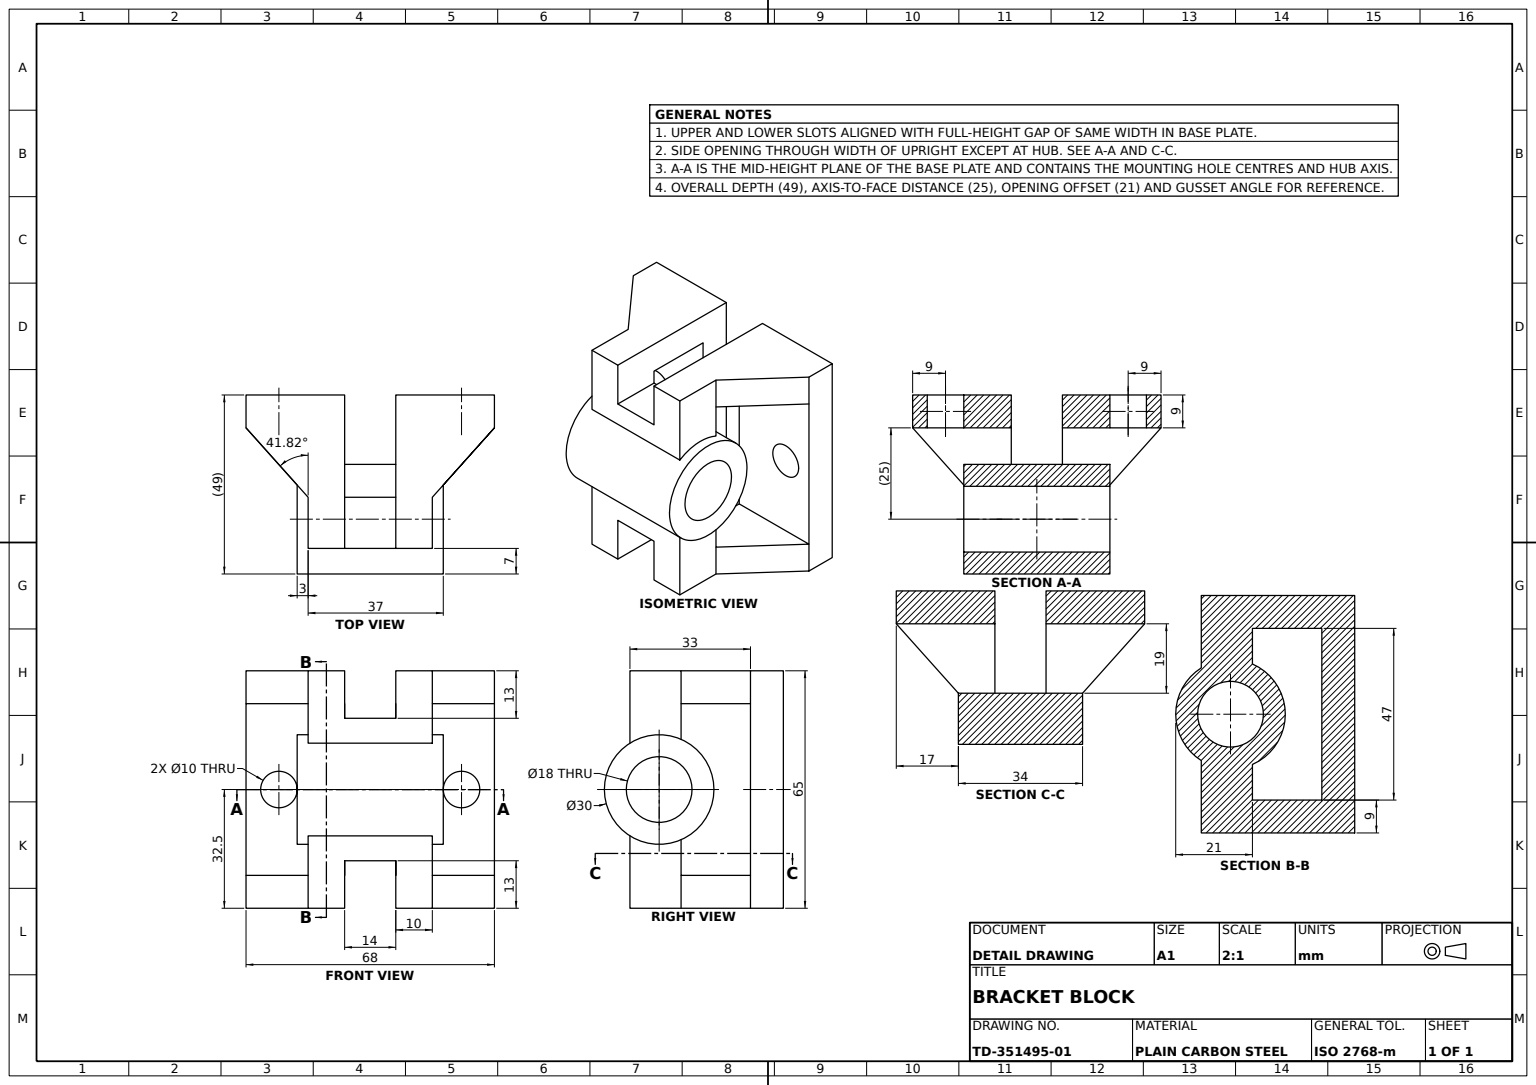
from build123d import *

# Parameters (mm, degrees)
BASE_PLATE_SKETCH_W        = 68
BASE_PLATE_SKETCH_H        = 65
BASE_PLATE_68X65_DEPTH     = 9
UPRIGHT_BLOCK_DEPTH        = 9
SECOND_UPRIGHT_BLOCK_DEPTH = 9
SIDE_WEB_SKETCH_W          = 34
SIDE_WEB_SKETCH_H          = 14
SIDE_WEB_DEPTH             = 65
UPPER_SLOT_7X14_DEPTH      = 13
LOWER_SLOT_7X14_DEPTH      = 13
THROUGH_CHANNEL_SKETCH_W   = 14
THROUGH_CHANNEL_SKETCH_H   = 9
THROUGH_CHANNEL_DEPTH      = 65
BEARING_HUB_SKETCH_R       = 15
BEARING_HUB_DEPTH          = 37
HUB_START                  = 3
HUB_COLLAR_SKETCH_30_R     = 15
HUB_COLLAR_30_DEPTH        = 3
CENTER_BORE_SKETCH_18_R    = 9
CENTER_BORE_18_DEPTH       = 65
SIDE_POCKET_SKETCH_R       = 5
SIDE_POCKET_CUT_DEPTH      = 9


with BuildPart() as part:
    # Base Plate Sketch → Base Plate 68x65 (new body)
    with BuildSketch(Plane.XY):
        with Locations((34, 32.5)):
            Rectangle(BASE_PLATE_SKETCH_W, BASE_PLATE_SKETCH_H)
    extrude(amount=BASE_PLATE_68X65_DEPTH)

    # Upright Block Sketch → Upright Block (add)
    with BuildSketch(Plane.XZ):
        Polygon((0, 9), (68, 9), (51, 28), (51, 42), (34, 42), (17, 42), (17, 28), align=None)
    extrude(amount=-UPRIGHT_BLOCK_DEPTH)

    # Second Upright Sketch → Second Upright Block (add)
    with BuildSketch(Plane(origin=(0, 65, 0), x_dir=(1, 0, 0), z_dir=(0, 1, 0))):
        Polygon((34, -42), (51, -42), (51, -28), (68, -9), (0, -9), (17, -28), (17, -42), align=None)
    extrude(amount=-SECOND_UPRIGHT_BLOCK_DEPTH)

    # Side Web Sketch → Side Web (add)
    with BuildSketch(Plane.XZ):
        with Locations((34, 35)):
            Rectangle(SIDE_WEB_SKETCH_W, SIDE_WEB_SKETCH_H)
    extrude(amount=-SIDE_WEB_DEPTH)

    # Upper Slot Sketch → Upper Slot 7x14 (cut)
    with BuildSketch(Plane.XZ):
        Polygon((34, 42), (41, 42), (41, 0), (27, 0), (27, 42), align=None)
    extrude(amount=-UPPER_SLOT_7X14_DEPTH, mode=Mode.SUBTRACT)

    # Lower Slot Sketch → Lower Slot 7x14 (cut)
    with BuildSketch(Plane(origin=(0, 65, 0), x_dir=(1, 0, 0), z_dir=(0, 1, 0))):
        Polygon((34, -42), (41, -42), (41, 0), (27, 0), (27, -42), align=None)
    extrude(amount=-LOWER_SLOT_7X14_DEPTH, mode=Mode.SUBTRACT)

    # Through Channel Sketch → Through Channel (cut)
    with BuildSketch(Plane.XZ.offset(-13)):
        with Locations((34, 4.5)):
            Rectangle(THROUGH_CHANNEL_SKETCH_W, THROUGH_CHANNEL_SKETCH_H)
    extrude(amount=-THROUGH_CHANNEL_DEPTH, mode=Mode.SUBTRACT)

    # Bearing Hub Sketch → Bearing Hub (add)
    with BuildSketch(Plane.ZY.offset(-17)):
        with Locations((34, 32.5)):
            Circle(BEARING_HUB_SKETCH_R)
    extrude(amount=-BEARING_HUB_DEPTH)

    # Hub Collar Sketch Ø30 → Hub Collar Ø30 (add)
    with BuildSketch(Plane.ZY.offset(-17).offset(HUB_START)):
        with Locations((34, 32.5)):
            Circle(HUB_COLLAR_SKETCH_30_R)
    extrude(amount=-HUB_COLLAR_30_DEPTH)

    # Center Bore Sketch Ø18 → Center Bore Ø18 (cut)
    with BuildSketch(Plane.ZY.offset(-14)):
        with Locations((34, 32.5)):
            Circle(CENTER_BORE_SKETCH_18_R)
    extrude(amount=-CENTER_BORE_18_DEPTH, mode=Mode.SUBTRACT)

    # Side Pocket Sketch → Side Pocket Cut (cut)
    with BuildSketch(Plane(origin=(0, 0, 0), x_dir=(-1, 0, 0), z_dir=(0, 0, -1))):
        with Locations((-59, 32.5)):
            Circle(SIDE_POCKET_SKETCH_R)
        with Locations((-9, 32.5)):
            Circle(SIDE_POCKET_SKETCH_R)
    extrude(amount=-SIDE_POCKET_CUT_DEPTH, mode=Mode.SUBTRACT)


solid = part.part
